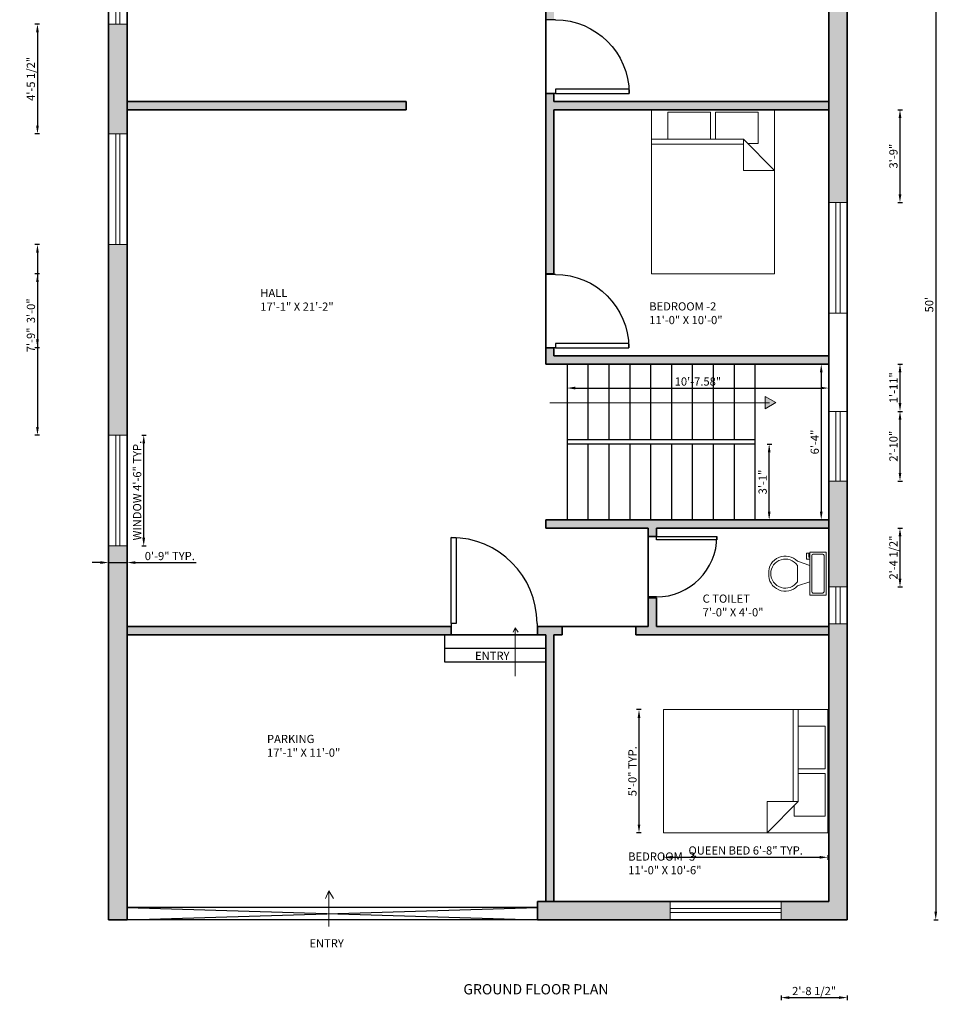
# Model space of a CAD drawing. Units: inches. Extents: x -40 to 407, y -627 to 108.
# Tile 1 of 2: x -40 to 407, y -627 to -147. Entities that reach past the tile are written whole.
import ezdxf

# ---------------------------------------------------------------- set-up
doc = ezdxf.new("R2010")
doc.units = ezdxf.units.IN
for name, color, linetype, lineweight in [('A-ANNO-DIMS', 2, 'Continuous', 18), ('A-ANNO-SYMB', 7, 'Continuous', 18), ('A-ANNO-TEXT', 7, 'Continuous', 18), ('A-AREA-IDEN', 7, 'Continuous', 18), ('A-DOOR', 4, 'Continuous', 25), ('A-FLOR-FIXT', 8, 'Continuous', 18), ('A-FLOR-STRS', 7, 'Continuous', 25), ('A-FURN', 8, 'Continuous', 18), ('A-GLAZ', 6, 'Continuous', 18), ('A-WALL', 7, 'Continuous', 35), ('A-WALL-PATT', 251, 'Continuous', 13)]:
    doc.layers.add(name, color=color, linetype=linetype, lineweight=lineweight)
doc.styles.get("Standard").update_dxf_attribs({"font": 'arial.ttf'})
doc.dimstyles.new('ISO-25', dxfattribs={"dimtxt": 4, "dimasz": 4, "dimexe": 1.25, "dimexo": 0.625, "dimtad": 1, "dimlunit": 3, "dimtxsty": 'Standard', "dimcen": 2.5, "dimadec": 0, "dimazin": 0, "dimtfac": 1, "dimtmove": 0, "dimatfit": 3, "dimfxl": 1, "dimfxlon": 1, "dimarcsym": 0})

# ---------------------------------------------------------------- blocks, each defined once
blk = doc.blocks.new('*U2')
for p, q in [((9.5, -6), (9.5, -2)), ((-10, -8.5), (-8, -8.5)), ((-10, -9.5), (-10, -8.5)), ((-7, -9.5), (-10, -9.5)), ((-8, -8.5), (-8, -8)), ((-7, -8), (-7, -9.5)), ((-4, -8), (-6, -14)), ((4, -8), (6, -14)), ((4, -14), (-4, -14))]:
    blk.add_line(p, q)
blk.add_lwpolyline([(10.5, -8), (10.5, 0), (-10.5, 0), (-10.5, -8)], close=True)
for points in [[(-9.5, -2), (-9.5, -6)], [(8.5, -1), (-8.5, -1)], [(-8.5, -7), (8.5, -7)]]:
    blk.add_lwpolyline(points)
for centre, radius, start, end in [((-8.625, -1.875), 0.8839, 81.8699, 188.1301), ((8.625, -1.875), 0.8839, 351.8699, 98.1301), ((-8.625, -6.125), 0.8839, 171.869898, 278.1301), ((8.625, -6.125), 0.8839, 261.8699, 8.1301), ((-0.4772, -19.9188), 8.0953, 133.01722, 273.38), ((0.0374, -19.8731), 7.127, 124.50543, 269.7), ((-0.0373, -19.8731), 7.127, 270.3, 55.4946), ((0.4773, -19.9188), 8.0953, 266.62, 46.9828)]:
    blk.add_arc(centre, radius, start, end)
blk = doc.blocks.new('*U4')
for p, q in [((0, 0), (0, -100)), ((750, 0), (750, -100))]:
    blk.add_line(p, q)
blk.add_lwpolyline([(0, 0), (0, 750), (43.75, 750), (43.75, 0)], close=True)
blk.add_arc((0, 0), 750, 0, 90)
blk = doc.blocks.new('Bed - Queen')
for p, q in [((0, -80.00003), (0, 0)), ((0, 0), (59.99999, 0)), ((59.99999, 0), (59.99999, -80.00003)), ((7.99999, -1.2), (28.79998, -1.2)), ((7.99999, -14.4), (7.99999, -1.2)), ((28.79998, -1.2), (28.79998, -14.4)), ((31.19999, -1.2), (51.99999, -1.2)), ((31.19999, -14.4), (31.19999, -1.2)), ((51.99999, -1.2), (51.99999, -16.4)), ((0, -14.4), (44.8, -14.4)), ((59.99999, -29.6), (44.8, -14.4)), ((44.8, -14.4), (44.8, -29.6)), ((44.8, -16.8), (0, -16.8)), ((51.99999, -16.4), (46.79936, -16.4)), ((44.8, -29.6), (59.99999, -29.6)), ((59.99999, -80.00003), (0, -80.00003))]:
    blk.add_line(p, q)
blk = doc.blocks.new('*D10')
at = {"layer": 'A-ANNO-DIMS', "color": 0, "lineweight": -2, "transparency": 16777216}
for p, q in [((226.54, -325.81), (226.54, -328.06)), ((354.12, -325.81), (354.12, -328.06)), ((230.54, -326.81), (350.12, -326.81))]:
    blk.add_line(p, q, dxfattribs=at)
at = {"layer": 'A-ANNO-DIMS', "color": 0, "transparency": 16777216}
for points in [[(230.54, -326.14), (230.54, -327.47), (226.54, -326.81)], [(350.12, -326.14), (350.12, -327.47), (354.12, -326.81)]]:
    blk.add_solid(points, dxfattribs=at)
at = {"layer": 'Defpoints', "color": 0, "transparency": 16777216}
for p in [(226.54, -315.12), (354.12, -315.12), (354.12, -326.81)]:
    blk.add_point(p, dxfattribs=at)
at = {"layer": 'A-ANNO-DIMS', "color": 0, "transparency": 16777216, "insert": (290.33, -324.14), "char_height": 4, "attachment_point": 5}
blk.add_mtext('10\'-7.58"', dxfattribs=at)
blk = doc.blocks.new('*D11')
at = {"layer": 'A-ANNO-DIMS', "color": 0, "lineweight": -2, "transparency": 16777216}
for p, q in [((351.44, -315.12), (349.19, -315.12)), ((350.44, -319.12), (350.44, -387.12)), ((351.44, -391.12), (349.19, -391.12))]:
    blk.add_line(p, q, dxfattribs=at)
at = {"layer": 'A-ANNO-DIMS', "color": 0, "transparency": 16777216}
for points in [[(349.78, -319.12), (351.11, -319.12), (350.44, -315.12)], [(349.78, -387.12), (351.11, -387.12), (350.44, -391.12)]]:
    blk.add_solid(points, dxfattribs=at)
at = {"layer": 'Defpoints', "color": 0, "transparency": 16777216}
for p in [(354.12, -315.12), (350.44, -391.12), (354.12, -391.12)]:
    blk.add_point(p, dxfattribs=at)
at = {"layer": 'A-ANNO-DIMS', "color": 0, "transparency": 16777216, "insert": (347.78, -353.12), "char_height": 4, "attachment_point": 5, "rotation": 90}
blk.add_mtext('6\'-4"', dxfattribs=at)
blk = doc.blocks.new('*D12')
at = {"layer": 'A-ANNO-DIMS', "color": 0, "lineweight": -2, "transparency": 16777216}
for p, q in [((324.06, -354.12), (326.31, -354.12)), ((325.06, -387.12), (325.06, -358.12)), ((324.06, -391.12), (326.31, -391.12))]:
    blk.add_line(p, q, dxfattribs=at)
at = {"layer": 'A-ANNO-DIMS', "color": 0, "transparency": 16777216}
for points in [[(324.4, -358.12), (325.73, -358.12), (325.06, -354.12)], [(324.4, -387.12), (325.73, -387.12), (325.06, -391.12)]]:
    blk.add_solid(points, dxfattribs=at)
at = {"layer": 'Defpoints', "color": 0, "transparency": 16777216}
for p in [(318.12, -354.12), (325.06, -354.12), (318.12, -391.12)]:
    blk.add_point(p, dxfattribs=at)
at = {"layer": 'A-ANNO-DIMS', "color": 0, "transparency": 16777216, "insert": (322.39, -372.62), "char_height": 4, "attachment_point": 5, "rotation": 90}
blk.add_mtext('3\'-1"', dxfattribs=at)
blk = doc.blocks.new('*D14')
at = {"layer": 'A-ANNO-DIMS', "color": 0, "lineweight": -2, "transparency": 16777216}
for p, q in [((405.24, 13.88), (407.49, 13.88)), ((406.24, 9.88), (406.24, -582.12)), ((405.24, -586.12), (407.49, -586.12))]:
    blk.add_line(p, q, dxfattribs=at)
at = {"layer": 'A-ANNO-DIMS', "color": 0, "transparency": 16777216}
for points in [[(405.57, 9.88), (406.91, 9.88), (406.24, 13.88)], [(405.57, -582.12), (406.91, -582.12), (406.24, -586.12)]]:
    blk.add_solid(points, dxfattribs=at)
at = {"layer": 'Defpoints', "color": 0, "transparency": 16777216}
for p in [(363.12, 13.88), (363.12, -586.12), (406.24, -586.12)]:
    blk.add_point(p, dxfattribs=at)
at = {"layer": 'A-ANNO-DIMS', "color": 0, "transparency": 16777216, "insert": (403.57, -286.12), "char_height": 4, "attachment_point": 5, "rotation": 90}
blk.add_mtext("50'", dxfattribs=at)
blk = doc.blocks.new('WIN-54IN')
for p, q in [((3.5, 54), (3.5, 0)), ((5.5, 54), (5.5, 0))]:
    blk.add_line(p, q)
blk.add_lwpolyline([(0, 54), (9, 54), (9, 0), (0, 0)], close=True)
blk = doc.blocks.new('WIN-18IN')
for p, q in [((18, 5.5), (0, 5.5)), ((18, 3.5), (0, 3.5))]:
    blk.add_line(p, q)
blk.add_lwpolyline([(0, 9), (18, 9), (18, 0), (0, 0)], close=True)
blk = doc.blocks.new('*D17')
at = {"layer": 'A-ANNO-DIMS', "color": 0, "lineweight": -2, "transparency": 16777216}
for p, q in [((19.22, -349.81), (21.47, -349.81)), ((20.22, -399.81), (20.22, -353.81)), ((19.22, -403.81), (21.47, -403.81))]:
    blk.add_line(p, q, dxfattribs=at)
at = {"layer": 'A-ANNO-DIMS', "color": 0, "transparency": 16777216}
for points in [[(19.55, -353.81), (20.89, -353.81), (20.22, -349.81)], [(19.55, -399.81), (20.89, -399.81), (20.22, -403.81)]]:
    blk.add_solid(points, dxfattribs=at)
at = {"layer": 'Defpoints', "color": 0, "transparency": 16777216}
for p in [(12.12, -349.81), (20.22, -349.81), (12.12, -403.81)]:
    blk.add_point(p, dxfattribs=at)
at = {"layer": 'A-ANNO-DIMS', "color": 0, "transparency": 16777216, "insert": (17.53, -376.81), "char_height": 4, "attachment_point": 5, "rotation": 90}
blk.add_mtext('WINDOW 4\'-6" TYP.', dxfattribs=at)
blk = doc.blocks.new('*D18')
at = {"layer": 'A-ANNO-DIMS', "color": 0, "lineweight": -2, "transparency": 16777216}
for p, q in [((-0.88, -411.91), (-4.88, -411.91)), ((3.12, -410.91), (3.12, -413.16)), ((3.12, -411.91), (12.12, -411.91)), ((12.12, -410.91), (12.12, -413.16)), ((16.12, -411.91), (45.75, -411.91))]:
    blk.add_line(p, q, dxfattribs=at)
at = {"layer": 'A-ANNO-DIMS', "color": 0, "transparency": 16777216}
for points in [[(-0.88, -411.24), (-0.88, -412.57), (3.12, -411.91)], [(16.12, -411.24), (16.12, -412.57), (12.12, -411.91)]]:
    blk.add_solid(points, dxfattribs=at)
at = {"layer": 'Defpoints', "color": 0, "transparency": 16777216}
for p in [(3.12, -403.81), (12.12, -403.81), (12.12, -411.91)]:
    blk.add_point(p, dxfattribs=at)
at = {"layer": 'A-ANNO-DIMS', "color": 0, "transparency": 16777216, "insert": (32.94, -409.24), "char_height": 4, "attachment_point": 5}
blk.add_mtext('0\'-9" TYP.', dxfattribs=at)
blk = doc.blocks.new('*D19')
at = {"layer": 'A-ANNO-DIMS', "color": 0, "lineweight": -2, "transparency": 16777216}
for p, q in [((273.61, -554.63), (273.61, -556.88)), ((277.61, -555.63), (349.61, -555.63)), ((353.61, -554.63), (353.61, -556.88))]:
    blk.add_line(p, q, dxfattribs=at)
at = {"layer": 'A-ANNO-DIMS', "color": 0, "transparency": 16777216}
for points in [[(277.61, -554.96), (277.61, -556.3), (273.61, -555.63)], [(349.61, -554.96), (349.61, -556.3), (353.61, -555.63)]]:
    blk.add_solid(points, dxfattribs=at)
at = {"layer": 'Defpoints', "color": 0, "transparency": 16777216}
for p in [(273.61, -543.63), (353.61, -543.63), (353.61, -555.63)]:
    blk.add_point(p, dxfattribs=at)
at = {"layer": 'A-ANNO-DIMS', "color": 0, "transparency": 16777216, "insert": (313.61, -552.81), "char_height": 4, "attachment_point": 5}
blk.add_mtext('QUEEN BED 6\'-8" TYP.', dxfattribs=at)
blk = doc.blocks.new('*D20')
at = {"layer": 'A-ANNO-DIMS', "color": 0, "lineweight": -2, "transparency": 16777216}
for p, q in [((262.61, -483.63), (260.36, -483.63)), ((261.61, -487.63), (261.61, -539.63)), ((262.61, -543.63), (260.36, -543.63))]:
    blk.add_line(p, q, dxfattribs=at)
at = {"layer": 'A-ANNO-DIMS', "color": 0, "transparency": 16777216}
for points in [[(260.94, -487.63), (262.27, -487.63), (261.61, -483.63)], [(260.94, -539.63), (262.27, -539.63), (261.61, -543.63)]]:
    blk.add_solid(points, dxfattribs=at)
at = {"layer": 'Defpoints', "color": 0, "transparency": 16777216}
for p in [(273.61, -483.63), (261.61, -543.63), (273.61, -543.63)]:
    blk.add_point(p, dxfattribs=at)
at = {"layer": 'A-ANNO-DIMS', "color": 0, "transparency": 16777216, "insert": (258.94, -513.63), "char_height": 4, "attachment_point": 5, "rotation": 90}
blk.add_mtext('5\'-0" TYP.', dxfattribs=at)
blk = doc.blocks.new('*D33')
at = {"layer": 'A-ANNO-DIMS', "color": 0, "lineweight": -2, "transparency": 16777216}
for p, q in [((-30.58, -271.12), (-32.83, -271.12)), ((-31.58, -275.12), (-31.58, -303.12)), ((-30.58, -307.12), (-32.83, -307.12))]:
    blk.add_line(p, q, dxfattribs=at)
at = {"layer": 'A-ANNO-DIMS', "color": 0, "transparency": 16777216}
for points in [[(-32.25, -275.12), (-30.91, -275.12), (-31.58, -271.12)], [(-32.25, -303.12), (-30.91, -303.12), (-31.58, -307.12)]]:
    blk.add_solid(points, dxfattribs=at)
at = {"layer": 'Defpoints', "color": 0, "transparency": 16777216}
for p in [(216.12, -271.12), (-31.58, -307.12), (216.12, -307.12)]:
    blk.add_point(p, dxfattribs=at)
at = {"layer": 'A-ANNO-DIMS', "color": 0, "transparency": 16777216, "insert": (-34.25, -289.12), "char_height": 4, "attachment_point": 5, "rotation": 90}
blk.add_mtext('3\'-0"', dxfattribs=at)
blk = doc.blocks.new('*D34')
at = {"layer": 'A-ANNO-DIMS', "color": 0, "lineweight": -2, "transparency": 16777216}
for p, q in [((170.1, 98.58), (170.1, 100.83)), ((212.1, 98.58), (212.1, 100.83)), ((174.1, 99.58), (208.1, 99.58))]:
    blk.add_line(p, q, dxfattribs=at)
at = {"layer": 'A-ANNO-DIMS', "color": 0, "transparency": 16777216}
for points in [[(174.1, 100.25), (174.1, 98.91), (170.1, 99.58)], [(208.1, 100.25), (208.1, 98.91), (212.1, 99.58)]]:
    blk.add_solid(points, dxfattribs=at)
at = {"layer": 'Defpoints', "color": 0, "transparency": 16777216}
for p in [(212.1, 99.58), (170.1, -443.12), (212.1, -443.12)]:
    blk.add_point(p, dxfattribs=at)
at = {"layer": 'A-ANNO-DIMS', "color": 0, "transparency": 16777216, "insert": (191.1, 102.25), "char_height": 4, "attachment_point": 5}
blk.add_mtext('3\'-6"', dxfattribs=at)
blk = doc.blocks.new('*D36')
at = {"layer": 'A-ANNO-DIMS', "color": 0, "lineweight": -2, "transparency": 16777216}
for p, q in [((-30.58, -149.31), (-32.83, -149.31)), ((-31.58, -153.31), (-31.58, -198.8)), ((-30.58, -202.8), (-32.83, -202.8))]:
    blk.add_line(p, q, dxfattribs=at)
at = {"layer": 'A-ANNO-DIMS', "color": 0, "transparency": 16777216}
for points in [[(-32.25, -153.31), (-30.91, -153.31), (-31.58, -149.31)], [(-32.25, -198.8), (-30.91, -198.8), (-31.58, -202.8)]]:
    blk.add_solid(points, dxfattribs=at)
at = {"layer": 'Defpoints', "color": 0, "transparency": 16777216}
for p in [(3.12, -149.31), (-31.58, -202.8), (3.12, -202.8)]:
    blk.add_point(p, dxfattribs=at)
at = {"layer": 'A-ANNO-DIMS', "color": 0, "transparency": 16777216, "insert": (-34.27, -176.05), "char_height": 4, "attachment_point": 5, "rotation": 90}
blk.add_mtext('4\'-5 1/2"', dxfattribs=at)
blk = doc.blocks.new('*D37')
at = {"layer": 'A-ANNO-DIMS', "color": 0, "lineweight": -2, "transparency": 16777216}
for p, q in [((-30.58, -256.8), (-32.83, -256.8)), ((-31.58, -260.8), (-31.58, -345.81)), ((-30.58, -349.81), (-32.83, -349.81))]:
    blk.add_line(p, q, dxfattribs=at)
at = {"layer": 'A-ANNO-DIMS', "color": 0, "transparency": 16777216}
for points in [[(-32.25, -260.8), (-30.91, -260.8), (-31.58, -256.8)], [(-32.25, -345.81), (-30.91, -345.81), (-31.58, -349.81)]]:
    blk.add_solid(points, dxfattribs=at)
at = {"layer": 'Defpoints', "color": 0, "transparency": 16777216}
for p in [(3.12, -256.8), (-31.58, -349.81), (3.12, -349.81)]:
    blk.add_point(p, dxfattribs=at)
at = {"layer": 'A-ANNO-DIMS', "color": 0, "transparency": 16777216, "insert": (-34.25, -303.3), "char_height": 4, "attachment_point": 5, "rotation": 90}
blk.add_mtext('7\'-9"', dxfattribs=at)
blk = doc.blocks.new('*D39')
at = {"layer": 'A-ANNO-DIMS', "color": 0, "lineweight": -2, "transparency": 16777216}
for p, q in [((387.82, -191.12), (390.07, -191.12)), ((388.82, -195.12), (388.82, -232.33)), ((387.82, -236.33), (390.07, -236.33))]:
    blk.add_line(p, q, dxfattribs=at)
at = {"layer": 'A-ANNO-DIMS', "color": 0, "transparency": 16777216}
for points in [[(388.15, -195.12), (389.49, -195.12), (388.82, -191.12)], [(388.15, -232.33), (389.49, -232.33), (388.82, -236.33)]]:
    blk.add_solid(points, dxfattribs=at)
at = {"layer": 'Defpoints', "color": 0, "transparency": 16777216}
for p in [(354.12, -191.12), (354.12, -236.33), (388.82, -236.33)]:
    blk.add_point(p, dxfattribs=at)
at = {"layer": 'A-ANNO-DIMS', "color": 0, "transparency": 16777216, "insert": (386.15, -213.72), "char_height": 4, "attachment_point": 5, "rotation": 90}
blk.add_mtext('3\'-9"', dxfattribs=at)
blk = doc.blocks.new('*D40')
at = {"layer": 'A-ANNO-DIMS', "color": 0, "lineweight": -2, "transparency": 16777216}
for p, q in [((387.82, -315.12), (390.07, -315.12)), ((388.82, -319.12), (388.82, -334.17)), ((387.82, -338.17), (390.07, -338.17))]:
    blk.add_line(p, q, dxfattribs=at)
at = {"layer": 'A-ANNO-DIMS', "color": 0, "transparency": 16777216}
for points in [[(388.15, -319.12), (389.49, -319.12), (388.82, -315.12)], [(388.15, -334.17), (389.49, -334.17), (388.82, -338.17)]]:
    blk.add_solid(points, dxfattribs=at)
at = {"layer": 'Defpoints', "color": 0, "transparency": 16777216}
for p in [(354.12, -315.12), (354.12, -338.17), (388.82, -338.17)]:
    blk.add_point(p, dxfattribs=at)
at = {"layer": 'A-ANNO-DIMS', "color": 0, "transparency": 16777216, "insert": (386.19, -326.65), "char_height": 4, "attachment_point": 5, "rotation": 90}
blk.add_mtext('1\'-11"', dxfattribs=at)
blk = doc.blocks.new('*D41')
at = {"layer": 'A-ANNO-DIMS', "color": 0, "lineweight": -2, "transparency": 16777216}
for p, q in [((387.82, -338.17), (390.07, -338.17)), ((388.82, -342.17), (388.82, -368.17)), ((387.82, -372.17), (390.07, -372.17))]:
    blk.add_line(p, q, dxfattribs=at)
at = {"layer": 'A-ANNO-DIMS', "color": 0, "transparency": 16777216}
for points in [[(388.15, -342.17), (389.49, -342.17), (388.82, -338.17)], [(388.15, -368.17), (389.49, -368.17), (388.82, -372.17)]]:
    blk.add_solid(points, dxfattribs=at)
at = {"layer": 'Defpoints', "color": 0, "transparency": 16777216}
for p in [(354.12, -338.17), (354.12, -372.17), (388.82, -372.17)]:
    blk.add_point(p, dxfattribs=at)
at = {"layer": 'A-ANNO-DIMS', "color": 0, "transparency": 16777216, "insert": (386.15, -355.17), "char_height": 4, "attachment_point": 5, "rotation": 90}
blk.add_mtext('2\'-10"', dxfattribs=at)
blk = doc.blocks.new('*D42')
at = {"layer": 'A-ANNO-DIMS', "color": 0, "lineweight": -2, "transparency": 16777216}
for p, q in [((387.82, -395.12), (390.07, -395.12)), ((388.82, -399.12), (388.82, -419.81)), ((387.82, -423.81), (390.07, -423.81))]:
    blk.add_line(p, q, dxfattribs=at)
at = {"layer": 'A-ANNO-DIMS', "color": 0, "transparency": 16777216}
for points in [[(388.15, -399.12), (389.49, -399.12), (388.82, -395.12)], [(388.15, -419.81), (389.49, -419.81), (388.82, -423.81)]]:
    blk.add_solid(points, dxfattribs=at)
at = {"layer": 'Defpoints', "color": 0, "transparency": 16777216}
for p in [(354.12, -395.12), (354.12, -423.81), (388.82, -423.81)]:
    blk.add_point(p, dxfattribs=at)
at = {"layer": 'A-ANNO-DIMS', "color": 0, "transparency": 16777216, "insert": (386.13, -409.46), "char_height": 4, "attachment_point": 5, "rotation": 90}
blk.add_mtext('2\'-4 1/2"', dxfattribs=at)
blk = doc.blocks.new('*D43')
at = {"layer": 'A-ANNO-DIMS', "color": 0, "lineweight": -2, "transparency": 16777216}
for p, q in [((330.84, -623.04), (330.84, -625.29)), ((334.84, -624.04), (359.12, -624.04)), ((363.12, -623.04), (363.12, -625.29))]:
    blk.add_line(p, q, dxfattribs=at)
at = {"layer": 'A-ANNO-DIMS', "color": 0, "transparency": 16777216}
for points in [[(334.84, -623.37), (334.84, -624.7), (330.84, -624.04)], [(359.12, -623.37), (359.12, -624.7), (363.12, -624.04)]]:
    blk.add_solid(points, dxfattribs=at)
at = {"layer": 'Defpoints', "color": 0, "transparency": 16777216}
for p in [(330.84, -586.12), (363.12, -586.12), (363.12, -624.04)]:
    blk.add_point(p, dxfattribs=at)
at = {"layer": 'A-ANNO-DIMS', "color": 0, "transparency": 16777216, "insert": (346.98, -621.34), "char_height": 4, "attachment_point": 5}
blk.add_mtext('2\'-8 1/2"', dxfattribs=at)

msp = doc.modelspace()

# ---------------------------------------------------------------- hatches: boundary and pattern name
at = {"layer": 'A-ANNO-SYMB'}
h = msp.add_hatch(color=256, dxfattribs=at)
h.dxf.hatch_style = 1
h.paths.add_polyline_path([(323.169, -336.943), (328.352, -333.921), (323.169, -330.943)])
at = {"layer": 'A-WALL-PATT'}
h = msp.add_hatch(color=256, dxfattribs=at)
h.dxf.hatch_style = 1
h.paths.add_polyline_path([(12.12, 4.879), (46.39, 4.879), (46.39, 13.879), (3.12, 13.879), (3.12, -95.306), (12.12, -95.306)])
h.paths.add_polyline_path([(150.38, 13.879), (100.39, 13.879), (100.39, 4.879), (144.12, 4.879), (148.12, 4.879), (150.38, 4.879)])
h.paths.add_polyline_path([(363.12, 13.879), (168.38, 13.879), (168.38, 4.879), (187.717, 4.879), (216.12, 4.879), (220.12, 4.879), (354.12, 4.879), (354.12, -46.69), (363.12, -46.69)])
h.paths.add_polyline_path([(148.12, 4.879), (144.12, 4.879), (144.12, -66.121), (148.12, -66.121), (216.12, -66.121), (216.12, -112.121), (148.12, -112.121), (148.12, -96.121), (144.12, -96.121), (144.12, -141.121), (148.12, -141.121), (148.12, -116.121), (216.12, -116.121), (216.12, -147.121), (220.12, -147.121), (220.12, -58.121), (216.12, -58.121), (216.12, -62.121), (148.12, -62.121)])
h.paths.add_polyline_path([(220.12, 4.879), (216.12, 4.879), (216.12, -28.121), (220.12, -28.121)], flags=17)
h.paths.add_polyline_path([(363.12, -100.69), (354.12, -100.69), (354.12, -236.329), (363.12, -236.329)])
h.paths.add_polyline_path([(354.12, -187.121), (220.12, -187.121), (220.12, -183.121), (216.12, -183.121), (216.12, -271.121), (220.12, -271.121), (220.12, -191.121), (354.12, -191.121)])
h.paths.add_polyline_path([(363.12, -441.809), (354.12, -441.809), (354.12, -577.121), (330.838, -577.121), (330.838, -586.121), (363.12, -586.121)])
h.paths.add_polyline_path([(363.12, -372.174), (354.12, -372.174), (354.12, -391.121), (354.12, -423.809), (363.12, -423.809)])
h.paths.add_polyline_path([(354.12, -443.121), (270.12, -443.121), (270.12, -429.121), (266.12, -429.121), (266.12, -443.121), (260.12, -443.121), (260.12, -447.121), (266.12, -447.121), (270.12, -447.121), (354.12, -447.121)])
h.paths.add_polyline_path([(354.12, -391.121), (216.12, -391.121), (216.12, -395.121), (266.12, -395.121), (266.12, -399.121), (270.12, -399.121), (270.12, -395.121), (354.12, -395.121)])
h.paths.add_polyline_path([(354.12, -311.121), (220.12, -311.121), (220.12, -307.121), (216.12, -307.121), (216.12, -315.121), (354.12, -315.121)])
h.paths.add_polyline_path([(170.105, -443.121), (12.12, -443.121), (12.12, -447.121), (170.105, -447.121)])
h.paths.add_polyline_path([(12.12, -403.805), (3.12, -403.805), (3.12, -586.121), (12.12, -586.121)])
h.paths.add_polyline_path([(220.12, -447.121), (224.12, -447.121), (224.12, -443.121), (220.12, -443.121), (216.12, -443.121), (212.105, -443.121), (212.105, -447.121), (216.12, -447.121), (216.12, -577.121), (220.12, -577.121)])
h.paths.add_polyline_path([(276.838, -577.121), (212.099, -577.121), (212.099, -586.121), (276.838, -586.121)])
h = msp.add_hatch(color=256, dxfattribs=at)
h.dxf.hatch_style = 1
h.paths.add_polyline_path([(12.12, -256.798), (3.12, -256.798), (3.12, -349.805), (12.12, -349.805)])
h.paths.add_polyline_path([(12.12, -149.306), (3.12, -149.306), (3.12, -202.798), (12.12, -202.798)])
h.paths.add_polyline_path([(148.12, -187.121), (12.12, -187.121), (12.12, -191.121), (148.12, -191.121)])

# ---------------------------------------------------------------- linework, layer by layer
at = {"layer": 'A-ANNO-SYMB'}
for p, q in [((218.177, -333.963), (325.187, -333.963)), ((201.291, -443.657), (200.208, -445.864)), ((201.291, -467.237), (201.291, -443.657)), ((201.291, -443.657), (202.756, -445.864)), ((110.401, -571.976), (108.882, -575.702)), ((110.401, -571.976), (112.631, -575.73)), ((110.401, -571.976), (110.401, -589.338))]:
    msp.add_line(p, q, dxfattribs=at)
msp.add_lwpolyline([(323.169, -330.943), (323.169, -336.943), (328.352, -333.921)], close=True, dxfattribs=at)
at = {"layer": 'A-DOOR'}
for p, q in [((212.099, -580.121), (12.12, -580.121)), ((12.12, -586.121), (212.099, -580.121)), ((12.12, -580.121), (212.099, -586.121)), ((212.099, -586.121), (12.12, -586.121))]:
    msp.add_line(p, q, dxfattribs=at)
at = {"layer": 'A-FLOR-STRS'}
for p, q in [((226.541, -315.121), (226.541, -391.121)), ((236.717, -315.121), (236.717, -352.121)), ((246.892, -315.121), (246.892, -352.121)), ((257.067, -315.121), (257.067, -352.121)), ((267.243, -315.121), (267.243, -352.121)), ((277.418, -315.121), (277.418, -352.121)), ((287.593, -315.121), (287.593, -352.121)), ((297.769, -315.121), (297.769, -352.121)), ((307.944, -315.121), (307.944, -352.121)), ((318.12, -315.121), (318.12, -391.121)), ((318.12, -315.121), (318.12, -391.121)), ((318.12, -352.121), (226.541, -352.121)), ((318.12, -354.121), (226.541, -354.121)), ((236.717, -354.121), (236.717, -391.121)), ((246.892, -354.121), (246.892, -391.121)), ((257.067, -354.121), (257.067, -391.121)), ((267.243, -354.121), (267.243, -391.121)), ((277.418, -354.121), (277.418, -391.121)), ((287.593, -354.121), (287.593, -391.121)), ((297.769, -354.121), (297.769, -391.121)), ((307.944, -354.121), (307.944, -391.121)), ((216.12, -453.777), (166.96, -453.777))]:
    msp.add_line(p, q, dxfattribs=at)
msp.add_lwpolyline([(166.96, -447.121), (216.12, -447.121), (216.12, -460.434), (166.96, -460.434)], close=True, dxfattribs=at)
at = {"layer": 'A-GLAZ'}
for p, q in [((357.62, -338.174), (357.62, -372.174)), ((359.62, -338.174), (359.62, -372.174))]:
    msp.add_line(p, q, dxfattribs=at)
msp.add_lwpolyline([(354.12, -338.174), (363.12, -338.174), (363.12, -372.174), (354.12, -372.174)], close=True, dxfattribs=at)
at = {"layer": 'A-WALL'}
for p, q in [((3.12, -586.121), (3.12, 13.879)), ((363.12, 13.879), (363.12, -586.121)), ((12.12, -586.121), (12.12, 4.879)), ((354.12, 4.879), (354.12, -315.121)), ((216.12, -315.121), (216.12, -116.121)), ((12.12, -187.121), (148.12, -187.121)), ((148.12, -191.121), (148.12, -187.121)), ((220.12, -183.121), (216.12, -183.121)), ((220.12, -187.121), (220.12, -183.121)), ((220.12, -187.121), (354.12, -187.121)), ((12.12, -191.121), (148.12, -191.121)), ((220.12, -191.121), (354.12, -191.121)), ((220.12, -271.121), (220.12, -191.121)), ((220.12, -271.121), (216.12, -271.121)), ((220.12, -307.121), (216.12, -307.121)), ((220.12, -311.121), (220.12, -307.121)), ((220.12, -311.121), (354.12, -311.121)), ((216.12, -315.121), (354.12, -315.121)), ((354.12, -315.121), (354.12, -391.121)), ((216.12, -391.121), (354.12, -391.121)), ((216.12, -395.121), (216.12, -391.121)), ((354.12, -391.121), (354.12, -577.121)), ((216.12, -395.121), (266.12, -395.121)), ((266.12, -395.121), (266.12, -443.121)), ((270.12, -395.121), (270.12, -399.121)), ((270.12, -395.121), (354.12, -395.121)), ((270.12, -399.121), (266.12, -399.121)), ((270.12, -429.121), (266.12, -429.121)), ((270.12, -429.121), (270.12, -443.121)), ((170.105, -443.121), (12.12, -443.121)), ((170.105, -447.121), (170.105, -443.121)), ((216.12, -443.121), (212.105, -443.121)), ((212.105, -447.121), (212.105, -443.121)), ((220.12, -443.121), (216.12, -443.121)), ((266.12, -443.121), (220.12, -443.121)), ((224.12, -447.121), (224.12, -443.121)), ((260.12, -447.121), (260.12, -443.121)), ((270.12, -443.121), (354.12, -443.121)), ((216.12, -447.121), (12.12, -447.121)), ((216.12, -577.121), (216.12, -447.121)), ((220.12, -577.121), (220.12, -447.121)), ((224.12, -447.121), (220.12, -447.121)), ((266.12, -447.121), (260.12, -447.121)), ((270.12, -447.121), (266.12, -447.121)), ((270.12, -447.121), (354.12, -447.121)), ((354.12, -577.121), (212.099, -577.121)), ((212.099, -577.121), (212.099, -586.121)), ((12.12, -586.121), (3.12, -586.121)), ((363.12, -586.121), (212.099, -586.121))]:
    msp.add_line(p, q, dxfattribs=at)

# ---------------------------------------------------------------- block references
at = {"layer": 'A-DOOR', "rotation": 270}
for p, xscale, yscale, zscale in [((220.903, -183.121), -0.0478338880450648, 0.0478338880450648, 0.0478338880450648), ((220.882, -307.121), -0.0476269249643901, 0.0476269249643901, 0.0476269249643901), ((270.088, -399.121), 0.0393700787401575, 0.0393700787401575, 0.0393700787401575)]:
    msp.add_blockref('*U4', p, dxfattribs=dict(at, xscale=xscale, yscale=yscale, zscale=zscale))
at = {"layer": 'A-DOOR', "xscale": 0.055766802320118, "yscale": 0.055766802320118, "zscale": 0.055766802320118}
msp.add_blockref('*U4', (170.105, -441.544), dxfattribs=at)
at = {"layer": 'A-FLOR-FIXT', "rotation": 270}
msp.add_blockref('*U2', (352.82, -417.293), dxfattribs=at)
at = {"layer": 'A-FURN'}
msp.add_blockref('Bed - Queen', (267.668, -191.121), dxfattribs=at)
at = {"layer": 'A-FURN', "rotation": 270}
msp.add_blockref('Bed - Queen', (353.607, -483.631), dxfattribs=at)
at = {"layer": 'A-GLAZ'}
for p in [(3.12, -149.306), (3.12, -256.799), (354.12, -290.329), (3.12, -403.805)]:
    msp.add_blockref('WIN-54IN', p, dxfattribs=at)
at = {"layer": 'A-GLAZ', "extrusion": (0, 0, -1), "zscale": -1, "rotation": 270.0000000000001}
msp.add_blockref('WIN-18IN', (-363.12, -423.808), dxfattribs=at)
at = {"layer": 'A-GLAZ', "rotation": 270.0000000000002}
msp.add_blockref('WIN-54IN', (276.837, -577.121), dxfattribs=at)

# ---------------------------------------------------------------- texts
at = {"layer": 'A-ANNO-TEXT', "attachment_point": 1}
for s, width, insert, char_height in [('ENTRY', 11.27453, (181.691, -455.337), 4), ('ENTRY', 33.71452, (100.95, -595.567), 4), ('GROUND FLOOR PLAN', 174.0223, (176.018, -617.471), 5)]:
    msp.add_mtext_dynamic_manual_height_columns(s, width=width, gutter_width=12.5, heights=[0], dxfattribs=dict(at, insert=insert, char_height=char_height))
at = {"layer": 'A-AREA-IDEN', "char_height": 4, "attachment_point": 1}
for s, width, insert in [('HALL\\P17\'-1" X 21\'-2"', 87.33409, (77.04, -278.428)), ('BEDROOM -2\\P11\'-0" X 10\'-0"', 58.6794, (266.606, -284.982)), ('C TOILET\\P7\'-0" X 4\'-0"', 30.57261, (292.614, -427.488)), ('PARKING\\P17\'-1" X 11\'-0"', 94.82755, (80.299, -495.912)), ('BEDROOM -3\\P11\'-0" X 10\'-6"', 86.30329, (256.344, -553.248))]:
    msp.add_mtext_dynamic_manual_height_columns(s, width=width, gutter_width=12.5, heights=[0], dxfattribs=dict(at, insert=insert))

# ---------------------------------------------------------------- dimensions: what is measured, and where the dimension line sits
at = {"layer": 'A-ANNO-DIMS'}
for base, p1, p2, override, picture, middle in [((212.105, 99.579), (170.105, -443.121), (212.105, -443.121), {"dimdec": 1, "dimlfac": 1, "dimrnd": 0, "dimzin": 1, "dimdsep": 46, "dimlunit": 4, "dimfrac": 2}, '*D34', (191.105, 102.248)), ((354.12, -326.805), (226.541, -315.121), (354.12, -315.121), {"dimclrd": 0, "dimclre": 0, "dimclrt": 0}, '*D10', (290.33, -324.138)), ((363.12, -624.038), (330.838, -586.121), (363.12, -586.121), {"dimdec": 1, "dimlfac": 1, "dimrnd": 0, "dimzin": 1, "dimdsep": 46, "dimlunit": 4, "dimfrac": 2}, '*D43', (346.979, -621.344))]:
    dim = msp.add_linear_dim(base=base, p1=p1, p2=p2, dimstyle='ISO-25', override=override, dxfattribs=at)
    dim.commit()
    dim.dimension.update_dxf_attribs({"geometry": picture, "text_midpoint": middle})
for base, p1, p2, angle, override, picture, middle in [((406.24, -586.121), (363.12, 13.879), (363.12, -586.121), 90, {"dimclrd": 0, "dimclre": 0, "dimclrt": 0}, '*D14', (403.573, -286.121)), ((-31.58, -202.798), (3.12, -149.306), (3.12, -202.798), 90, {"dimdec": 1, "dimlfac": 1, "dimrnd": 0, "dimzin": 1, "dimdsep": 46, "dimlunit": 4, "dimfrac": 2}, '*D36', (-34.274, -176.052)), ((388.82, -236.329), (354.12, -191.121), (354.12, -236.329), 270, {"dimdec": 1, "dimlfac": 1, "dimrnd": 0, "dimzin": 1, "dimdsep": 46, "dimlunit": 4, "dimfrac": 2}, '*D39', (386.151, -213.725)), ((-31.58, -349.805), (3.12, -256.798), (3.12, -349.805), 90, {"dimdec": 1, "dimlfac": 1, "dimrnd": 0, "dimzin": 1, "dimdsep": 46, "dimlunit": 4, "dimfrac": 2}, '*D37', (-34.248, -303.302)), ((-31.58, -307.121), (216.12, -271.121), (216.12, -307.121), 90, {"dimdec": 1, "dimlfac": 1, "dimrnd": 0, "dimzin": 1, "dimdsep": 46, "dimlunit": 4, "dimfrac": 2}, '*D33', (-34.249, -289.121)), ((350.443, -391.121), (354.12, -315.121), (354.12, -391.121), 90, {"dimclrd": 0, "dimclre": 0, "dimclrt": 0}, '*D11', (347.775, -353.121)), ((388.82, -338.174), (354.12, -315.121), (354.12, -338.174), 270, {"dimdec": 1, "dimlfac": 1, "dimrnd": 0, "dimzin": 1, "dimdsep": 46, "dimlunit": 4, "dimfrac": 2}, '*D40', (386.186, -326.647)), ((388.82, -372.174), (354.12, -338.174), (354.12, -372.174), 270, {"dimdec": 1, "dimlfac": 1, "dimrnd": 0, "dimzin": 1, "dimdsep": 46, "dimlunit": 4, "dimfrac": 2}, '*D41', (386.152, -355.174)), ((325.064, -354.121), (318.12, -391.121), (318.12, -354.121), 90, {"dimclrd": 0, "dimclre": 0, "dimclrt": 0}, '*D12', (322.395, -372.621)), ((388.82, -423.809), (354.12, -395.121), (354.12, -423.809), 270, {"dimdec": 1, "dimlfac": 1, "dimrnd": 0, "dimzin": 1, "dimdsep": 46, "dimlunit": 4, "dimfrac": 2}, '*D42', (386.126, -409.465))]:
    dim = msp.add_linear_dim(base=base, p1=p1, p2=p2, angle=angle, dimstyle='ISO-25', override=override, dxfattribs=at)
    dim.commit()
    dim.dimension.update_dxf_attribs({"geometry": picture, "text_midpoint": middle})
for base, p1, p2, angle, text, picture, middle in [((20.22, -349.805), (12.12, -403.805), (12.12, -349.805), 90, 'WINDOW <> TYP.', '*D17', (17.525, -376.805)), ((261.607, -543.631), (273.607, -483.631), (273.607, -543.631), 270, '<> TYP.', '*D20', (258.939, -513.631))]:
    dim = msp.add_linear_dim(base=base, p1=p1, p2=p2, angle=angle, text=text, dimstyle='ISO-25', override={"dimdec": 1, "dimlfac": 1, "dimrnd": 0, "dimzin": 1, "dimdsep": 46, "dimlunit": 4, "dimfrac": 2}, dxfattribs=at)
    dim.commit()
    dim.dimension.update_dxf_attribs({"geometry": picture, "text_midpoint": middle})
for base, p1, p2, text, picture, middle in [((12.12, -411.905), (3.12, -403.805), (12.12, -403.805), '<> TYP.', '*D18', (32.936, -409.238)), ((353.607, -555.631), (273.607, -543.631), (353.607, -543.631), 'QUEEN BED <> TYP.', '*D19', (313.607, -552.815))]:
    dim = msp.add_linear_dim(base=base, p1=p1, p2=p2, text=text, dimstyle='ISO-25', override={"dimdec": 1, "dimlfac": 1, "dimrnd": 0, "dimzin": 1, "dimdsep": 46, "dimlunit": 4, "dimfrac": 2}, dxfattribs=at)
    dim.commit()
    dim.dimension.update_dxf_attribs({"geometry": picture, "text_midpoint": middle})

doc.saveas('drawing.dxf')
